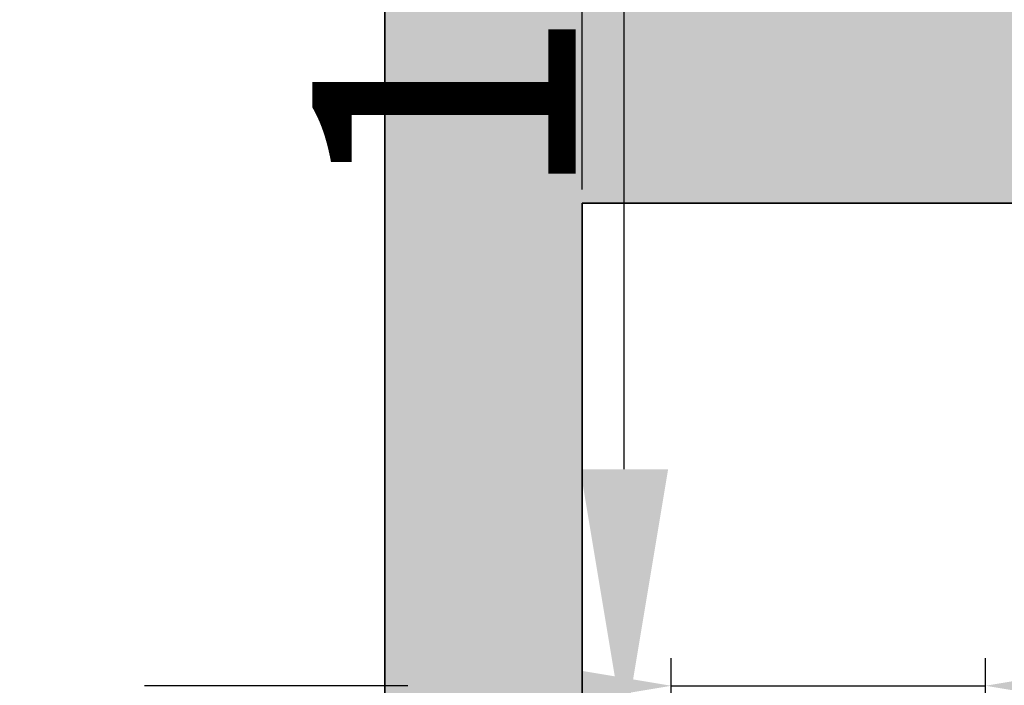
# Model space of a CAD drawing. Units: inches. Extents: x 2083 to 3317, y 1141 to 2115.
# Tile 16 of 256: x 2210 to 2255, y 1447 to 1477. Entities that reach past the tile are written whole.
import ezdxf

# ---------------------------------------------------------------- set-up
doc = ezdxf.new("R2010")
doc.units = ezdxf.units.IN
doc.layers.add('A-ANNO-DIMS', color=2, linetype='Continuous', lineweight=18)
doc.layers.add('A-WALL', color=7, linetype='Continuous', lineweight=35)
doc.layers.add('A-WALL-PATT', color=251, linetype='Continuous', lineweight=13, true_color=0x636466)
doc.styles.get("Standard").update_dxf_attribs({"font": 'arial.ttf'})
doc.dimstyles.new('ISO-25', dxfattribs={"dimtxt": 12, "dimasz": 12, "dimexe": 1.25, "dimexo": 0.625, "dimtad": 1, "dimlunit": 3, "dimtxsty": 'Standard', "dimcen": 2.5, "dimadec": 0, "dimazin": 0, "dimtfac": 1, "dimtmove": 0, "dimatfit": 3, "dimfxl": 1, "dimarcsym": 0})

# ---------------------------------------------------------------- blocks, each defined once
blk = doc.blocks.new('*D13')
at = {"layer": 'A-ANNO-DIMS', "color": 0, "lineweight": -2, "transparency": 16777216}
for p, q in [((2226.335, 1477.761), (2191.976, 1477.761)), ((2193.226, 1465.761), (2193.226, 1275.261)), ((2226.335, 1263.261), (2191.976, 1263.261))]:
    blk.add_line(p, q, dxfattribs=at)
at = {"layer": 'A-ANNO-DIMS', "color": 0, "transparency": 16777216}
for points in [[(2191.226, 1465.761), (2195.226, 1465.761), (2193.226, 1477.761)], [(2191.226, 1275.261), (2195.226, 1275.261), (2193.226, 1263.261)]]:
    blk.add_solid(points, dxfattribs=at)
at = {"layer": 'Defpoints', "color": 0, "transparency": 16777216}
for p in [(2226.96, 1477.761), (2193.226, 1263.261), (2226.96, 1263.261)]:
    blk.add_point(p, dxfattribs=at)
at = {"layer": 'A-ANNO-DIMS', "color": 0, "transparency": 16777216, "insert": (2186.474, 1370.511), "char_height": 12, "attachment_point": 5, "rotation": 90}
blk.add_mtext('17\'-10.5"', dxfattribs=at)
blk = doc.blocks.new('*D30')
at = {"layer": 'A-ANNO-DIMS', "color": 0, "lineweight": -2, "transparency": 16777216}
for p, q in [((2240.018, 1445.274), (2240.018, 1448.046)), ((2254.329, 1445.274), (2254.329, 1448.046)), ((2228.018, 1446.796), (2216.018, 1446.796)), ((2240.018, 1446.796), (2254.329, 1446.796)), ((2266.329, 1446.796), (2413.765, 1446.796))]:
    blk.add_line(p, q, dxfattribs=at)
at = {"layer": 'A-ANNO-DIMS', "color": 0, "transparency": 16777216}
for points in [[(2228.018, 1448.796), (2228.018, 1444.796), (2240.018, 1446.796)], [(2266.329, 1448.796), (2266.329, 1444.796), (2254.329, 1446.796)]]:
    blk.add_solid(points, dxfattribs=at)
at = {"layer": 'Defpoints', "color": 0, "transparency": 16777216}
for p in [(2254.329, 1446.796), (2240.018, 1444.649), (2254.329, 1444.649)]:
    blk.add_point(p, dxfattribs=at)
at = {"layer": 'A-ANNO-DIMS', "color": 0, "transparency": 16777216, "insert": (2346.047, 1453.625), "char_height": 12, "attachment_point": 5}
blk.add_mtext('WC 1\'-2 1/2" TYP.', dxfattribs=at)
blk = doc.blocks.new('*D31')
at = {"layer": 'A-ANNO-DIMS', "color": 0, "lineweight": -2, "transparency": 16777216}
for p, q in [((2237.871, 1456.649), (2237.871, 1541.915)), ((2239.393, 1444.649), (2236.621, 1444.649)), ((2237.871, 1431.548), (2237.871, 1444.649)), ((2239.393, 1431.548), (2236.621, 1431.548)), ((2237.871, 1419.548), (2237.871, 1407.548))]:
    blk.add_line(p, q, dxfattribs=at)
at = {"layer": 'A-ANNO-DIMS', "color": 0, "transparency": 16777216}
for points in [[(2235.871, 1456.649), (2239.871, 1456.649), (2237.871, 1444.649)], [(2235.871, 1419.548), (2239.871, 1419.548), (2237.871, 1431.548)]]:
    blk.add_solid(points, dxfattribs=at)
at = {"layer": 'Defpoints', "color": 0, "transparency": 16777216}
for p in [(2237.871, 1444.649), (2240.018, 1444.649), (2240.018, 1431.548)]:
    blk.add_point(p, dxfattribs=at)
at = {"layer": 'A-ANNO-DIMS', "color": 0, "transparency": 16777216, "insert": (2231.217, 1505.282), "char_height": 12, "attachment_point": 5, "rotation": 90}
blk.add_mtext('1\'-1" TYP.', dxfattribs=at)
blk = doc.blocks.new('*D62')
at = {"layer": 'A-ANNO-DIMS', "color": 0, "lineweight": -2, "transparency": 16777216}
for p, q in [((2235.96, 1469.386), (2235.96, 1522.361)), ((2379.96, 1469.386), (2379.96, 1522.361)), ((2247.96, 1521.111), (2367.96, 1521.111))]:
    blk.add_line(p, q, dxfattribs=at)
at = {"layer": 'A-ANNO-DIMS', "color": 0, "transparency": 16777216}
for points in [[(2247.96, 1523.111), (2247.96, 1519.111), (2235.96, 1521.111)], [(2367.96, 1523.111), (2367.96, 1519.111), (2379.96, 1521.111)]]:
    blk.add_solid(points, dxfattribs=at)
at = {"layer": 'Defpoints', "color": 0, "transparency": 16777216}
for p in [(2379.96, 1521.111), (2235.96, 1468.761), (2379.96, 1468.761)]:
    blk.add_point(p, dxfattribs=at)
at = {"layer": 'A-ANNO-DIMS', "color": 0, "transparency": 16777216, "insert": (2307.96, 1527.863), "char_height": 12, "attachment_point": 5}
blk.add_mtext('12\'-0"', dxfattribs=at)

msp = doc.modelspace()

# ---------------------------------------------------------------- hatches: boundary and pattern name
at = {"layer": 'A-WALL-PATT'}
h = msp.add_hatch(color=256, dxfattribs=at)
h.dxf.hatch_style = 1
h.paths.add_polyline_path([(3126.96, 2020.761), (2748.96, 2020.761), (2604.96, 2020.761), (2226.96, 2020.761), (2226.96, 1702.761), (2466.96, 1702.761), (2466.96, 1582.761), (2418.96, 1582.761), (2418.96, 1477.761), (2226.96, 1477.761), (2226.96, 1263.261), (2544.96, 1263.261), (2544.96, 1411.761), (2604.96, 1411.761), (2685.96, 1411.761), (2685.96, 1420.761), (2604.96, 1420.761), (2604.96, 1573.761), (2604.96, 1702.761), (2604.96, 2011.761), (2748.96, 2011.761), (2748.96, 1702.761), (2862.96, 1702.761), (2862.96, 1621.761), (2871.96, 1621.761), (2871.96, 1702.761), (2883.96, 1702.761), (2883.96, 1706.939, -0.026459), (2883.96, 1711.761), (2757.96, 1711.761), (2757.96, 1807.761), (2787.96, 1807.761), (2787.96, 1812.261), (2757.96, 1812.261), (2757.96, 2011.761), (2877.96, 2011.761), (2877.96, 1812.261), (2847.96, 1812.261), (2847.96, 1807.761), (2889.836, 1807.761), (2889.836, 1812.261), (2882.46, 1812.261), (2882.46, 2011.761), (3117.96, 2011.761), (3117.96, 1812.261), (2937.836, 1812.261), (2937.836, 1807.761), (2995.71, 1807.761), (2995.71, 1796.118), (3000.21, 1796.118), (3000.21, 1807.761), (3117.96, 1807.761), (3117.96, 1711.761), (3000.21, 1711.761), (3000.21, 1760.118), (2998.573, 1760.118, -0.020711), (2995.71, 1760.118), (2995.71, 1711.761), (2931.96, 1711.761), (2931.96, 1702.761), (3126.96, 1702.761)])
h.paths.add_polyline_path([(2471.46, 2011.761), (2471.46, 1810.011), (2462.717, 1810.011), (2462.717, 1805.511), (2505.96, 1805.511), (2505.96, 1810.011), (2475.96, 1810.011), (2475.96, 2011.761), (2595.96, 2011.761), (2595.96, 1810.011), (2565.96, 1810.011), (2565.96, 1805.511), (2595.96, 1805.511), (2595.96, 1711.761), (2235.96, 1711.761), (2235.96, 1805.511), (2353.71, 1805.511), (2353.71, 1796.054), (2358.21, 1796.054), (2358.21, 1805.511), (2414.717, 1805.511), (2414.717, 1810.011), (2235.96, 1810.011), (2235.96, 2011.761)], flags=16)
h.paths.add_polyline_path([(2270.205, 1994.61), (2270.205, 1970.61), (2246.205, 1970.61), (2246.205, 1994.61)], flags=0)
edge = h.paths.add_edge_path(flags=0)
edge.add_ellipse((2332.027, 1899.798), major_axis=(-3.043, 3.043), ratio=0.168252, start_angle=-161.3322, end_angle=-156.3071, ccw=False)
edge.add_ellipse((2333.082, 1898.744), major_axis=(-1.055, 1.055), ratio=0.453532, start_angle=-123.371, end_angle=-94.1591)
edge = h.paths.add_edge_path(flags=0)
edge.add_ellipse((2332.027, 1968.876), major_axis=(3.043, 3.043), ratio=0.168252, start_angle=18.6678, end_angle=23.6929)
edge.add_spline(control_points=[(2332.926, 1970.691), (2332.227, 1970.336), (2330.894, 1969.659), (2328.413, 1970.932), (2327.204, 1967.749), (2324.71, 1969.956), (2322.533, 1967.012), (2320.013, 1971.296), (2317.68, 1968.158), (2316.041, 1967.102), (2315.427, 1966.81)], knot_values=[0, 0, 0, 0, 2.267059, 4.324559, 6.685584, 8.878641, 11.121502, 14.300359, 17.755284, 19.732645, 19.732645, 19.732645, 19.732645], degree=3, periodic=0)
edge.add_ellipse((2332.027, 1968.876), major_axis=(3.043, 3.043), ratio=0.168252, start_angle=18.6678, end_angle=23.6929, ccw=False)
edge.add_ellipse((2333.082, 1969.931), major_axis=(1.055, 1.055), ratio=0.453532, start_angle=56.629, end_angle=85.8409, ccw=False)
edge = h.paths.add_edge_path(flags=0)
edge.add_spline(control_points=[(2296.428, 1967.988), (2293.628, 1965.336), (2287.704, 1959.727), (2299.744, 1949.996), (2294.533, 1935.669), (2290.573, 1920.604), (2293.394, 1909.974), (2296.185, 1904.967)], knot_values=[0.099185, 0.099185, 0.099185, 0.099185, 0.345301, 0.619822, 0.982653, 1.386093, 1.810555, 1.810555, 1.810555, 1.810555], degree=3, periodic=0)
edge.add_spline(control_points=[(2296.185, 1904.967), (2297.384, 1902.619), (2298.001, 1901.949), (2298.553, 1901.468)], knot_values=[0.006246, 0.006246, 0.006246, 0.006246, 0.055476, 0.055476, 0.055476, 0.055476], degree=3, periodic=0)
edge.add_spline(control_points=[(2298.553, 1901.468), (2297.259, 1900.923), (2295.225, 1900.232), (2293.06, 1900.614), (2292.101, 1900.788), (2292.09, 1900.791)], knot_values=[0.312835, 0.312835, 0.312835, 0.312835, 0.40178, 0.474987, 0.475903, 0.475903, 0.475903, 0.475903], degree=3, periodic=0)
edge.add_arc((2292.794, 1904.664), 3.937, 215.4209, 259.6982, ccw=False)
edge.add_spline(control_points=[(2289.585, 1902.382), (2289.477, 1902.535), (2289.368, 1902.688), (2289.261, 1902.841)], knot_values=[0.102872, 0.102872, 0.102872, 0.102872, 0.116896, 0.116896, 0.116896, 0.116896], degree=3, periodic=0)
edge.add_spline(control_points=[(2289.261, 1902.841), (2288.687, 1902.55), (2287.64, 1902.02), (2285.881, 1901.874), (2283.853, 1901.504), (2281.72, 1899.711), (2278.467, 1899.493), (2276.157, 1901.883), (2272.259, 1899.804), (2267.778, 1901.843), (2262.244, 1900.184), (2257.415, 1901.782), (2254.318, 1900.726), (2253.178, 1900.337)], knot_values=[0, 0, 0, 0, 1.907977, 3.477176, 5.261074, 7.972851, 11.680248, 13.717921, 16.939592, 22.789562, 27.502503, 33.595215, 37.145618, 37.145618, 37.145618, 37.145618], degree=3, periodic=0)
edge.add_line((2253.178, 1900.337), (2250.244, 1902.841))
edge.add_line((2250.244, 1902.841), (2250.244, 1965.833))
edge.add_line((2250.244, 1965.833), (2253.178, 1968.337))
edge.add_spline(control_points=[(2253.178, 1968.337), (2254.318, 1967.948), (2257.415, 1966.892), (2262.244, 1968.49), (2267.778, 1966.831), (2271.527, 1968.537), (2273.876, 1967.828), (2274.207, 1967.728)], knot_values=[0, 0, 0, 0, 0.09018, 0.244935, 0.364644, 0.513233, 0.537855, 0.537855, 0.537855, 0.537855], degree=3, periodic=0)
edge.add_arc((2274.353, 1963.793), 3.937, 72.0511, 92.1279, ccw=False)
edge.add_arc((2281.297, 1985.23), 18.596, 252.0511, 288.5657)
edge.add_arc((2292.317, 1956.029), 12.646, 71.0268, 113.7782, ccw=False)
edge = h.paths.add_edge_path(flags=0)
edge.add_spline(control_points=[(2274.899, 1951.856), (2275.066, 1951.617), (2275.233, 1951.377), (2275.398, 1951.136)], knot_values=[1.409916, 1.409916, 1.409916, 1.409916, 1.43159, 1.43159, 1.43159, 1.43159], degree=3, periodic=0)
edge.add_spline(control_points=[(2275.398, 1951.136), (2275.792, 1950.562), (2276.179, 1949.984), (2276.546, 1949.397)], knot_values=[1.358238, 1.358238, 1.358238, 1.358238, 1.409916, 1.409916, 1.409916, 1.409916], degree=3, periodic=0)
edge.add_line((2276.546, 1949.397), (2277.437, 1947.862))
edge.add_spline(control_points=[(2277.437, 1947.862), (2276.304, 1945.673), (2274.64, 1942.427), (2274.632, 1938.094), (2272.799, 1930.852), (2274.356, 1943.897), (2275.948, 1947.923), (2276.546, 1949.397)], knot_values=[0.005632, 0.005632, 0.005632, 0.005632, 0.186014, 0.266002, 0.357087, 0.59639, 0.739732, 0.739732, 0.739732, 0.739732], degree=3, periodic=0)
edge.add_spline(control_points=[(2276.546, 1949.397), (2276.179, 1949.984), (2275.792, 1950.562), (2275.398, 1951.136)], knot_values=[1.358238, 1.358238, 1.358238, 1.358238, 1.409916, 1.409916, 1.409916, 1.409916], degree=3, periodic=0)
edge.add_spline(control_points=[(2275.398, 1951.136), (2274.943, 1950.08), (2274.208, 1948.025), (2273.935, 1944.851), (2272.469, 1937.627), (2273.466, 1945.696), (2274.701, 1951.059), (2274.899, 1951.856)], knot_values=[0.104364, 0.104364, 0.104364, 0.104364, 0.189636, 0.269624, 0.36071, 0.600013, 0.644622, 0.644622, 0.644622, 0.644622], degree=3, periodic=0)
h.paths.add_polyline_path([(2269.168, 1963.128, -0.357527), (2268.171, 1960.976, -0.092561), (2268.171, 1939.436, -0.357527), (2269.168, 1937.285, -0.357527), (2267.016, 1938.282, -0.164785), (2254.686, 1938.282, -0.357527), (2252.534, 1937.285, -0.357527), (2253.531, 1939.436, -0.092561), (2253.531, 1960.976, -0.357527), (2252.534, 1963.128, -0.357527), (2254.686, 1962.131, -0.164785), (2267.016, 1962.131, -0.357527)], flags=0)
h.paths.add_polyline_path([(2248.874, 1967.802), (2248.874, 1957.028), (2249.458, 1957.028), (2249.458, 1911.647), (2248.874, 1911.647), (2248.874, 1900.873), (2246.512, 1900.873, 0.197327), (2244.15, 1902.457), (2244.15, 1966.218, 0.197327), (2246.512, 1967.802)], flags=0)
h.paths.add_polyline_path([(2269.168, 1931.389, -0.357527), (2268.171, 1929.238, -0.092561), (2268.171, 1907.698, -0.357527), (2269.168, 1905.547, -0.357527), (2267.016, 1906.544, -0.164785), (2254.686, 1906.544, -0.357527), (2252.534, 1905.547, -0.357527), (2253.531, 1907.698, -0.092561), (2253.531, 1929.238, -0.357527), (2252.534, 1931.389, -0.357527), (2254.686, 1930.392, -0.164785), (2267.016, 1930.392, -0.357527)], flags=0)
edge = h.paths.add_edge_path(flags=0)
edge.add_spline(control_points=[(2276.197, 1906.724), (2276.168, 1909.029), (2276.114, 1913.372), (2270.598, 1924.925), (2273.905, 1919.013), (2275.922, 1916.262), (2275.475, 1912.402), (2277.258, 1910.381), (2276.696, 1908.225), (2276.646, 1906.813), (2276.618, 1906.008)], knot_values=[0, 0, 0, 0, 8.61026, 16.221274, 18.843057, 23.804898, 27.440828, 29.356102, 31.203478, 33.650687, 33.650687, 33.650687, 33.650687], degree=3, periodic=0)
edge.add_spline(control_points=[(2276.618, 1906.008), (2276.623, 1905.624), (2276.498, 1904.629), (2275.442, 1903.855), (2274.937, 1903.08), (2274.859, 1902.841)], knot_values=[0.156488, 0.156488, 0.156488, 0.156488, 0.184398, 0.231376, 0.250598, 0.250598, 0.250598, 0.250598], degree=3, periodic=0)
edge.add_line((2274.859, 1902.841), (2276.506, 1902.841))
edge.add_spline(control_points=[(2276.506, 1902.841), (2276.788, 1903.085), (2277.665, 1904.125), (2278.25, 1904.341), (2277.654, 1908.527), (2278.156, 1906.228), (2278.1, 1905.286), (2278.847, 1904.069), (2277.857, 1903.415), (2277.874, 1902.991), (2277.904, 1902.841)], knot_values=[0.059574, 0.059574, 0.059574, 0.059574, 0.080753, 0.103741, 0.16972, 0.176036, 0.207137, 0.240474, 0.262341, 0.27366, 0.27366, 0.27366, 0.27366], degree=3, periodic=0)
edge.add_line((2277.904, 1902.841), (2280.03, 1902.841))
edge.add_spline(control_points=[(2280.03, 1902.841), (2279.888, 1903.088), (2279.499, 1903.982), (2280.152, 1905.939), (2278.104, 1909.658), (2279.762, 1907.185), (2280.328, 1904.875), (2280.485, 1903.49), (2281.463, 1903.249), (2281.758, 1902.936), (2281.834, 1902.841)], knot_values=[0.013856, 0.013856, 0.013856, 0.013856, 0.034874, 0.088867, 0.107879, 0.126738, 0.158714, 0.193757, 0.217487, 0.226722, 0.226722, 0.226722, 0.226722], degree=3, periodic=0)
edge.add_spline(control_points=[(2281.834, 1902.841), (2281.788, 1902.827), (2281.647, 1902.783), (2281.396, 1902.859), (2281.088, 1902.985), (2280.721, 1903.061), (2280.333, 1903.026), (2280.125, 1902.899), (2280.03, 1902.841)], knot_values=[0, 0, 0, 0, 0.14413, 0.435517, 0.749276, 1.153046, 1.548371, 1.878348, 1.878348, 1.878348, 1.878348], degree=3, periodic=0)
edge.add_line((2280.03, 1902.841), (2277.904, 1902.841))
edge.add_spline(control_points=[(2277.904, 1902.841), (2277.893, 1902.796), (2277.865, 1902.68), (2277.607, 1902.687), (2277.274, 1902.801), (2276.838, 1902.62), (2276.584, 1902.789), (2276.506, 1902.841)], knot_values=[0, 0, 0, 0, 0.127189, 0.326199, 0.628009, 1.24357, 1.515331, 1.515331, 1.515331, 1.515331], degree=3, periodic=0)
edge.add_line((2276.506, 1902.841), (2274.859, 1902.841))
edge.add_spline(control_points=[(2274.859, 1902.841), (2274.814, 1902.899), (2274.725, 1903.013), (2274.493, 1903.119), (2274.244, 1902.961), (2273.937, 1903.185), (2273.614, 1902.983), (2273.408, 1902.883), (2273.322, 1902.841)], knot_values=[0, 0, 0, 0, 0.21843, 0.436957, 0.687977, 0.990379, 1.398396, 1.69185, 1.69185, 1.69185, 1.69185], degree=3, periodic=0)
edge.add_spline(control_points=[(2273.322, 1902.841), (2273.617, 1903.446), (2274.274, 1904.538), (2276.027, 1904.574), (2276.207, 1906.584), (2276.197, 1906.724)], knot_values=[0.012227, 0.012227, 0.012227, 0.012227, 0.059472, 0.106218, 0.134458, 0.134458, 0.134458, 0.134458], degree=3, periodic=0)
h.paths.add_polyline_path([(2270.776, 1897.79), (2270.776, 1873.79), (2246.776, 1873.79), (2246.776, 1897.79)], flags=0)
h.paths.add_polyline_path([(2353.71, 1760.005), (2353.71, 1760.054), (2358.21, 1760.054, -0.033729)], flags=0)
h.paths.add_polyline_path([(2321.819, 1737.529), (2341.995, 1737.529, -0.414214), (2343.203, 1736.321), (2343.203, 1721.021, -0.414214), (2341.995, 1719.813), (2321.819, 1719.813, -0.414214), (2320.611, 1721.021), (2320.611, 1736.321, -0.414214)], flags=0)
h.paths.add_polyline_path([(2324.235, 1736.321), (2339.579, 1736.321, -0.414214), (2341.995, 1733.905), (2341.995, 1725.45, -0.414214), (2339.579, 1723.034), (2333.681, 1723.034), (2333.845, 1722.045, -0.870646), (2335.425, 1721.826, -0.767327), (2333.923, 1721.423), (2331.291, 1721.423, -0.767327), (2329.788, 1721.826, -0.870646), (2331.368, 1722.045), (2331.533, 1723.034), (2324.235, 1723.034, -0.414214), (2321.819, 1725.45), (2321.819, 1733.905, -0.414214)], flags=0)
h.paths.add_polyline_path([(2570.484, 1928.615), (2589.684, 1928.615), (2590.169, 1928.615), (2590.169, 1904.993), (2570.484, 1904.993)], flags=0)
h.paths.add_polyline_path([(2574.447, 1927.264, -1), (2572.829, 1927.264, -1)], flags=0)
h.paths.add_polyline_path([(2573.09, 1926.941), (2573.925, 1927.776), (2574.148, 1927.553), (2573.313, 1926.718)], flags=0)
h.paths.add_polyline_path([(2578.779, 1919.73, -1), (2571.592, 1919.73, -1)], flags=0)
h.paths.add_polyline_path([(2578.385, 1919.73, -1), (2571.985, 1919.73, -1)], flags=0)
h.paths.add_polyline_path([(2331.596, 1729.476, -1), (2333.618, 1729.476, -1)], flags=0)
h.paths.add_polyline_path([(2578.034, 1927.264, -1), (2576.416, 1927.264, -1)], flags=0)
h.paths.add_polyline_path([(2576.689, 1927.531), (2576.912, 1927.754), (2577.747, 1926.919), (2577.524, 1926.696)], flags=0)
h.paths.add_polyline_path([(2578.139, 1909.86, -1), (2572.232, 1909.86, -1)], flags=0)
h.paths.add_polyline_path([(2577.745, 1909.86, -1), (2572.625, 1909.86, -1)], flags=0)
h.paths.add_polyline_path([(2583.798, 1927.264, -1), (2582.179, 1927.264, -1)], flags=0)
h.paths.add_polyline_path([(2582.719, 1927.754), (2583.554, 1926.919), (2583.331, 1926.696), (2582.496, 1927.531)], flags=0)
h.paths.add_polyline_path([(2582.496, 1927.531), (2582.719, 1927.754), (2583.554, 1926.919), (2583.331, 1926.696)], flags=0)
h.paths.add_polyline_path([(2587.739, 1920.53, -1), (2581.832, 1920.53, -1)], flags=0)
h.paths.add_polyline_path([(2587.345, 1920.53, -1), (2582.225, 1920.53, -1)], flags=0)
h.paths.add_polyline_path([(2587.385, 1927.264, -1), (2585.766, 1927.264, -1)], flags=0)
h.paths.add_polyline_path([(2586.082, 1926.98), (2586.917, 1927.815), (2587.14, 1927.593), (2586.305, 1926.758)], flags=0)
h.paths.add_polyline_path([(2588.379, 1910.66, -1), (2581.192, 1910.66, -1)], flags=0)
h.paths.add_polyline_path([(2587.985, 1910.66, -1), (2581.585, 1910.66, -1)], flags=0)
h.paths.add_polyline_path([(2417.168, 1729.478), (2437.344, 1729.478, -0.414214), (2438.552, 1728.27), (2438.552, 1712.969, -0.414214), (2437.344, 1711.761), (2417.168, 1711.761, -0.414214), (2415.96, 1712.969), (2415.96, 1728.27, -0.414214)], flags=0)
h.paths.add_polyline_path([(2419.584, 1728.27), (2434.928, 1728.27, -0.414214), (2437.344, 1725.854), (2437.344, 1717.398, -0.414214), (2434.928, 1714.983), (2429.029, 1714.983), (2429.194, 1713.994, -0.870646), (2430.774, 1713.775, -0.767327), (2429.271, 1713.372), (2426.64, 1713.372, -0.767327), (2425.137, 1713.775, -0.870646), (2426.717, 1713.994), (2426.882, 1714.983), (2419.584, 1714.983, -0.414214), (2417.168, 1717.398), (2417.168, 1725.854, -0.414214)], flags=0)
h.paths.add_polyline_path([(2419.584, 1728.27), (2434.928, 1728.27, -0.414214), (2437.344, 1725.854), (2437.344, 1717.398, -0.414214), (2434.928, 1714.983), (2429.029, 1714.983), (2428.358, 1719.009), (2427.553, 1719.009), (2426.882, 1714.983), (2419.584, 1714.983, -0.414214), (2417.168, 1717.398), (2417.168, 1725.854, -0.414214)], flags=0)
h.paths.add_polyline_path([(2426.944, 1721.425, -1), (2428.967, 1721.425, -1)], flags=0)
h.paths.add_polyline_path([(2475.96, 1702.761), (2595.96, 1702.761), (2595.96, 1582.761), (2475.96, 1582.761)], flags=16)
h.paths.add_polyline_path([(2427.96, 1573.761), (2595.96, 1573.761), (2595.96, 1468.761), (2595.96, 1420.761), (2384.46, 1420.761), (2384.46, 1468.761), (2427.96, 1468.761)], flags=16)
h.paths.add_polyline_path([(2379.96, 1468.761), (2379.96, 1420.761), (2235.96, 1420.761), (2235.96, 1468.761)], flags=16)
h.paths.add_polyline_path([(2317.816, 1466.696), (2337.992, 1466.696, -0.414214), (2339.2, 1465.488), (2339.2, 1450.187, -0.414214), (2337.992, 1448.979), (2317.816, 1448.979, -0.414214), (2316.608, 1450.187), (2316.608, 1465.488, -0.414214)], flags=0)
h.paths.add_polyline_path([(2320.232, 1465.488), (2335.576, 1465.488, -0.414214), (2337.992, 1463.072), (2337.992, 1454.616, -0.414214), (2335.576, 1452.2), (2329.677, 1452.2), (2329.842, 1451.212, -0.870646), (2331.422, 1450.992, -0.767327), (2329.92, 1450.59), (2327.288, 1450.59, -0.767327), (2325.785, 1450.992, -0.870646), (2327.365, 1451.212), (2327.53, 1452.2), (2320.232, 1452.2, -0.414214), (2317.816, 1454.616), (2317.816, 1463.072, -0.414214)], flags=0)
h.paths.add_polyline_path([(2320.232, 1465.488), (2335.576, 1465.488, -0.414214), (2337.992, 1463.072), (2337.992, 1454.616, -0.414214), (2335.576, 1452.2), (2329.677, 1452.2), (2329.006, 1456.227), (2328.201, 1456.227), (2327.53, 1452.2), (2320.232, 1452.2, -0.414214), (2317.816, 1454.616), (2317.816, 1463.072, -0.414214)], flags=0)
h.paths.add_polyline_path([(2327.593, 1458.643, -1), (2329.615, 1458.643, -1)], flags=0)
h.paths.add_polyline_path([(2244.412, 1433.34), (2241.921, 1433.34, -0.414214), (2240.018, 1435.244), (2240.018, 1440.953, -0.414211), (2241.921, 1442.856), (2244.412, 1442.856, -1.976472)], flags=0)
h.paths.add_polyline_path([(2245.357, 1434.398, -0.414214), (2245.357, 1441.799, -2.144098)], flags=0)
h.paths.add_polyline_path([(2535.96, 1416.261), (2535.96, 1272.261), (2235.96, 1272.261), (2235.96, 1416.261)], flags=16)
h.paths.add_polyline_path([(2260.12, 1384.293), (2260.12, 1362.039), (2237.865, 1362.039), (2237.865, 1384.293)], flags=0)
edge = h.paths.add_edge_path(flags=0)
edge.add_line((2318.252, 1362.093), (2318.146, 1362.001))
edge.add_ellipse((2317.445, 1360.431), major_axis=(2.822, 2.822), ratio=0.168252, start_angle=18.6678, end_angle=20.9481, ccw=False)
edge.add_ellipse((2318.423, 1361.409), major_axis=(0.978, 0.978), ratio=0.453532, start_angle=56.629, end_angle=70.2262, ccw=False)
edge = h.paths.add_edge_path(flags=0)
edge.add_line((2319.107, 1295.571), (2319.015, 1295.677))
edge.add_ellipse((2317.445, 1296.378), major_axis=(-2.822, 2.822), ratio=0.168252, start_angle=-161.3322, end_angle=-159.0519, ccw=False)
edge.add_ellipse((2318.423, 1295.4), major_axis=(-0.978, 0.978), ratio=0.453532, start_angle=-123.371, end_angle=-109.7738)
edge = h.paths.add_edge_path(flags=0)
edge.add_spline(control_points=[(2284.21, 1301.17), (2284.581, 1300.445), (2284.891, 1299.892), (2285.16, 1299.461)], knot_values=[0.039066, 0.039066, 0.039066, 0.039066, 0.055476, 0.055476, 0.055476, 0.055476], degree=3, periodic=0)
edge.add_line((2285.16, 1299.461), (2284.21, 1301.17))
edge = h.paths.add_edge_path(flags=0)
edge.add_line((2280.412, 1297.298), (2283.37, 1297.036))
edge.add_line((2283.37, 1297.036), (2286.406, 1297.926))
edge.add_spline(control_points=[(2286.406, 1297.926), (2285.305, 1297.463), (2284.345, 1297.129), (2283.37, 1297.036)], knot_values=[0.394369, 0.394369, 0.394369, 0.394369, 0.475903, 0.475903, 0.475903, 0.475903], degree=3, periodic=0)
edge.add_spline(control_points=[(2283.37, 1297.036), (2283.281, 1297.028), (2282.316, 1296.957), (2281.313, 1297.134), (2280.423, 1297.296), (2280.412, 1297.298)], knot_values=[0.312835, 0.312835, 0.312835, 0.312835, 0.320246, 0.393453, 0.394369, 0.394369, 0.394369, 0.394369], degree=3, periodic=0)
edge = h.paths.add_edge_path(flags=0)
edge.add_line((2284.436, 1359.607), (2280.446, 1355.328))
edge.add_line((2280.446, 1355.328), (2279.58, 1351.018))
edge.add_line((2279.58, 1351.018), (2282.413, 1346.58))
edge.add_spline(control_points=[(2282.413, 1346.58), (2283.153, 1345.589), (2284.253, 1344.029), (2284.801, 1342.387), (2284.935, 1341.806)], knot_values=[1.240098, 1.240098, 1.240098, 1.240098, 1.332892, 1.382712, 1.382712, 1.382712, 1.382712], degree=3, periodic=0)
edge.add_spline(control_points=[(2284.935, 1341.806), (2285.319, 1340.141), (2285.233, 1338.409), (2284.91, 1336.654)], knot_values=[1.097484, 1.097484, 1.097484, 1.097484, 1.240098, 1.240098, 1.240098, 1.240098], degree=3, periodic=0)
edge.add_spline(control_points=[(2284.91, 1336.654), (2284.587, 1334.899), (2284.027, 1333.12), (2283.463, 1331.361)], knot_values=[0.95487, 0.95487, 0.95487, 0.95487, 1.097484, 1.097484, 1.097484, 1.097484], degree=3, periodic=0)
edge.add_line((2283.463, 1331.361), (2281.89, 1326.153))
edge.add_line((2281.89, 1326.153), (2280.756, 1321.056))
edge.add_line((2280.756, 1321.056), (2280.299, 1316.002))
edge.add_line((2280.299, 1316.002), (2280.716, 1310.95))
edge.add_line((2280.716, 1310.95), (2282.028, 1305.972))
edge.add_line((2282.028, 1305.972), (2284.21, 1301.17))
edge.add_spline(control_points=[(2284.21, 1301.17), (2283.341, 1302.73), (2282.612, 1304.336), (2282.028, 1305.972)], knot_values=[0.099185, 0.099185, 0.099185, 0.099185, 0.241799, 0.241799, 0.241799, 0.241799], degree=3, periodic=0)
edge.add_spline(control_points=[(2282.028, 1305.972), (2281.444, 1307.608), (2281.005, 1309.273), (2280.716, 1310.95)], knot_values=[0.241799, 0.241799, 0.241799, 0.241799, 0.384413, 0.384413, 0.384413, 0.384413], degree=3, periodic=0)
edge.add_spline(control_points=[(2280.716, 1310.95), (2280.433, 1312.588), (2280.289, 1314.277), (2280.299, 1315.962), (2280.299, 1316.002)], knot_values=[0.384413, 0.384413, 0.384413, 0.384413, 0.523647, 0.527028, 0.527028, 0.527028, 0.527028], degree=3, periodic=0)
edge.add_spline(control_points=[(2280.299, 1316.002), (2280.312, 1317.687), (2280.478, 1319.368), (2280.756, 1321.056)], knot_values=[0.527028, 0.527028, 0.527028, 0.527028, 0.669642, 0.669642, 0.669642, 0.669642], degree=3, periodic=0)
edge.add_spline(control_points=[(2280.756, 1321.056), (2281.035, 1322.744), (2281.426, 1324.44), (2281.89, 1326.153)], knot_values=[0.669642, 0.669642, 0.669642, 0.669642, 0.812256, 0.812256, 0.812256, 0.812256], degree=3, periodic=0)
edge.add_spline(control_points=[(2281.89, 1326.153), (2282.264, 1327.533), (2282.788, 1329.262), (2283.353, 1331.018), (2283.463, 1331.361)], knot_values=[0.812256, 0.812256, 0.812256, 0.812256, 0.927087, 0.95487, 0.95487, 0.95487, 0.95487], degree=3, periodic=0)
edge.add_line((2283.463, 1331.361), (2284.91, 1336.654))
edge.add_line((2284.91, 1336.654), (2284.935, 1341.806))
edge.add_line((2284.935, 1341.806), (2282.413, 1346.58))
edge.add_spline(control_points=[(2282.413, 1346.58), (2281.275, 1348.104), (2280.078, 1349.57), (2279.58, 1351.018)], knot_values=[1.382712, 1.382712, 1.382712, 1.382712, 1.525326, 1.525326, 1.525326, 1.525326], degree=3, periodic=0)
edge.add_spline(control_points=[(2279.58, 1351.018), (2279.443, 1351.415), (2279.136, 1352.857), (2279.735, 1354.29), (2280.446, 1355.328)], knot_values=[1.525326, 1.525326, 1.525326, 1.525326, 1.564439, 1.667941, 1.667941, 1.667941, 1.667941], degree=3, periodic=0)
edge.add_spline(control_points=[(2280.446, 1355.328), (2281.426, 1356.758), (2282.931, 1358.183), (2284.436, 1359.607)], knot_values=[1.667941, 1.667941, 1.667941, 1.667941, 1.810555, 1.810555, 1.810555, 1.810555], degree=3, periodic=0)
edge.add_arc((2280.623, 1348.518), 11.726, 71.0268, 113.7782)
edge.add_arc((2270.405, 1375.595), 17.244, 252.0511, 288.5657, ccw=False)
edge.add_arc((2263.966, 1355.718), 3.651, 72.0511, 92.1279)
edge.add_arc((2263.966, 1355.718), 3.651, 92.1279, 177.9851)
edge.add_spline(control_points=[(2260.318, 1355.846), (2260.26, 1354.221), (2260.551, 1350.187), (2262.999, 1346.766), (2264.473, 1344.649)], knot_values=[1.43159, 1.43159, 1.43159, 1.43159, 1.564144, 1.770695, 1.770695, 1.770695, 1.770695], degree=3, periodic=0)
edge.add_line((2264.473, 1344.649), (2264.936, 1343.983))
edge.add_spline(control_points=[(2263.801, 1340.248), (2263.843, 1340.514), (2264.067, 1341.756), (2264.513, 1343.002), (2264.935, 1343.981)], knot_values=[0.53657, 0.53657, 0.53657, 0.53657, 0.559349, 0.644622, 0.644622, 0.644622, 0.644622], degree=3, periodic=0)
edge.add_spline(control_points=[(2264.935, 1343.981), (2265.118, 1343.715), (2265.299, 1343.448), (2265.477, 1343.179)], knot_values=[1.384077, 1.384077, 1.384077, 1.384077, 1.409916, 1.409916, 1.409916, 1.409916], degree=3, periodic=0)
edge.add_spline(control_points=[(2265.477, 1343.179), (2265.655, 1342.911), (2265.829, 1342.641), (2265.999, 1342.369)], knot_values=[1.358238, 1.358238, 1.358238, 1.358238, 1.384077, 1.384077, 1.384077, 1.384077], degree=3, periodic=0)
edge.add_line((2265.999, 1342.369), (2266.826, 1340.946))
edge.add_spline(control_points=[(2266.826, 1340.946), (2268.894, 1337.09), (2271.398, 1325.843), (2270.516, 1310.569), (2275.919, 1301.861), (2277.79, 1299.199)], knot_values=[0.116896, 0.116896, 0.116896, 0.116896, 0.472987, 1.050969, 1.313793, 1.313793, 1.313793, 1.313793], degree=3, periodic=0)
edge.add_spline(control_points=[(2277.79, 1299.199), (2277.839, 1299.128), (2277.889, 1299.057), (2277.94, 1298.987)], knot_values=[0.109884, 0.109884, 0.109884, 0.109884, 0.116896, 0.116896, 0.116896, 0.116896], degree=3, periodic=0)
edge.add_line((2277.94, 1298.987), (2277.789, 1299.199))
edge.add_spline(control_points=[(2277.789, 1299.199), (2277.257, 1298.929), (2276.286, 1298.438), (2275.039, 1298.334), (2274.383, 1298.239), (2274.215, 1298.209)], knot_values=[33.12187, 33.12187, 33.12187, 33.12187, 35.029056, 36.598255, 37.144827, 37.144827, 37.144827, 37.144827], degree=3, periodic=0)
edge.add_line((2274.215, 1298.209), (2273.073, 1297.893))
edge.add_spline(control_points=[(2273.073, 1297.893), (2272.323, 1297.58), (2271.039, 1296.511), (2269.248, 1296.226), (2268.423, 1296.375)], knot_values=[26.532584, 26.532584, 26.532584, 26.532584, 29.198919, 31.839101, 31.839101, 31.839101, 31.839101], degree=3, periodic=0)
edge.add_line((2268.423, 1296.375), (2263.879, 1297.458))
edge.add_spline(control_points=[(2263.879, 1297.458), (2263.556, 1297.359), (2261.86, 1296.839), (2260.239, 1297.282), (2258.933, 1297.516)], knot_values=[15.919551, 15.919551, 15.919551, 15.919551, 16.939592, 21.226067, 21.226067, 21.226067, 21.226067], degree=3, periodic=0)
edge.add_line((2258.933, 1297.516), (2254.055, 1297.329))
edge.add_spline(control_points=[(2254.055, 1297.329), (2253.756, 1297.296), (2252.114, 1297.165), (2250.462, 1297.544), (2249.13, 1297.668)], knot_values=[5.306517, 5.306517, 5.306517, 5.306517, 6.276435, 10.613034, 10.613034, 10.613034, 10.613034], degree=3, periodic=0)
edge.add_line((2249.13, 1297.668), (2244.332, 1296.878))
edge.add_line((2244.332, 1296.878), (2241.611, 1299.199))
edge.add_line((2241.611, 1299.199), (2241.611, 1357.609))
edge.add_line((2241.611, 1357.609), (2244.332, 1359.931))
edge.add_line((2244.332, 1359.931), (2252.729, 1359.543))
edge.add_spline(control_points=[(2252.729, 1359.543), (2252.871, 1359.546), (2253.306, 1359.548), (2253.74, 1359.514), (2254.032, 1359.482)], knot_values=[0.233291, 0.233291, 0.233291, 0.233291, 0.244935, 0.268927, 0.268927, 0.268927, 0.268927], degree=3, periodic=0)
edge.add_line((2254.032, 1359.482), (2259.587, 1359.416))
edge.add_spline(control_points=[(2259.587, 1359.416), (2260.677, 1359.629), (2262.073, 1359.897), (2263.524, 1359.459), (2263.83, 1359.366)], knot_values=[0.422516, 0.422516, 0.422516, 0.422516, 0.513233, 0.537855, 0.537855, 0.537855, 0.537855], degree=3, periodic=0)
edge.add_arc((2263.966, 1355.718), 3.651, 72.0511, 92.1279, ccw=False)
edge.add_arc((2270.405, 1375.595), 17.244, 252.0511, 288.5657)
edge.add_arc((2280.623, 1348.518), 11.726, 71.0268, 113.7782, ccw=False)
h.paths.add_polyline_path([(2240.341, 1359.435), (2240.341, 1349.444), (2240.882, 1349.444), (2240.882, 1307.365), (2240.341, 1307.365), (2240.341, 1297.374), (2238.15, 1297.374, 0.197327), (2235.96, 1298.843), (2235.96, 1357.966, 0.197327), (2238.15, 1359.435)], flags=0)
h.paths.add_polyline_path([(2259.158, 1355.101, -0.357527), (2258.233, 1353.106, -0.092561), (2258.233, 1333.133, -0.357527), (2259.158, 1331.138, -0.357527), (2257.163, 1332.062, -0.164785), (2245.729, 1332.062, -0.357527), (2243.735, 1331.138, -0.357527), (2244.659, 1333.133, -0.092561), (2244.659, 1353.106, -0.357527), (2243.735, 1355.101, -0.357527), (2245.729, 1354.176, -0.164785), (2257.163, 1354.176, -0.357527)], flags=0)
edge = h.paths.add_edge_path(flags=0)
edge.add_line((2265.999, 1342.369), (2266.826, 1340.946))
edge.add_line((2266.826, 1340.946), (2265.308, 1337.814))
edge.add_line((2265.308, 1337.814), (2264.358, 1334.653))
edge.add_line((2264.358, 1334.653), (2264.262, 1333.8))
edge.add_spline(control_points=[(2264.262, 1333.8), (2264.208, 1333.187), (2264.162, 1332.366), (2264.007, 1331.414), (2263.969, 1331.202)], knot_values=[0.464444, 0.464444, 0.464444, 0.464444, 0.516691, 0.531608, 0.531608, 0.531608, 0.531608], degree=3, periodic=0)
edge.add_spline(control_points=[(2263.969, 1331.202), (2263.775, 1330.119), (2263.424, 1328.791), (2263.257, 1328.531), (2263.234, 1328.515)], knot_values=[0.372682, 0.372682, 0.372682, 0.372682, 0.44885, 0.464444, 0.464444, 0.464444, 0.464444], degree=3, periodic=0)
edge.add_spline(control_points=[(2263.234, 1328.515), (2263.096, 1328.42), (2263.131, 1329.301), (2263.275, 1330.616)], knot_values=[0.280919, 0.280919, 0.280919, 0.280919, 0.372682, 0.372682, 0.372682, 0.372682], degree=3, periodic=0)
edge.add_spline(control_points=[(2263.275, 1330.616), (2263.419, 1331.93), (2263.672, 1333.677), (2263.97, 1335.315)], knot_values=[0.189157, 0.189157, 0.189157, 0.189157, 0.280919, 0.280919, 0.280919, 0.280919], degree=3, periodic=0)
edge.add_spline(control_points=[(2263.97, 1335.315), (2264.1, 1336.032), (2264.419, 1337.622), (2264.755, 1338.864), (2264.947, 1339.491)], knot_values=[0.097394, 0.097394, 0.097394, 0.097394, 0.137578, 0.189157, 0.189157, 0.189157, 0.189157], degree=3, periodic=0)
edge.add_spline(control_points=[(2264.947, 1339.491), (2265.29, 1340.606), (2265.644, 1341.494), (2265.999, 1342.369)], knot_values=[0.005632, 0.005632, 0.005632, 0.005632, 0.097394, 0.097394, 0.097394, 0.097394], degree=3, periodic=0)
h.paths.add_polyline_path([(2259.158, 1325.671, -0.357527), (2258.233, 1323.676, -0.092561), (2258.233, 1303.703, -0.357527), (2259.158, 1301.708, -0.357527), (2257.163, 1302.633, -0.164785), (2245.729, 1302.633, -0.357527), (2243.735, 1301.708, -0.357527), (2244.659, 1303.703, -0.092561), (2244.659, 1323.676, -0.357527), (2243.735, 1325.671, -0.357527), (2245.729, 1324.747, -0.164785), (2257.163, 1324.747, -0.357527)], flags=0)
edge = h.paths.add_edge_path(flags=0)
edge.add_spline(control_points=[(2261.709, 1317.311), (2261.679, 1317.418), (2261.762, 1317.389), (2262.491, 1316.09), (2262.962, 1315.301)], knot_values=[14.955861, 14.955861, 14.955861, 14.955861, 16.221274, 18.694826, 18.694826, 18.694826, 18.694826], degree=3, periodic=0)
edge.add_spline(control_points=[(2262.962, 1315.301), (2262.99, 1315.254), (2263.702, 1314.067), (2264.349, 1313.127), (2264.73, 1312.164)], knot_values=[18.694826, 18.694826, 18.694826, 18.694826, 18.843057, 22.433791, 22.433791, 22.433791, 22.433791], degree=3, periodic=0)
edge.add_spline(control_points=[(2264.73, 1312.164), (2264.876, 1311.796), (2265.177, 1310.77), (2265.143, 1309.559), (2265.248, 1308.824)], knot_values=[22.433791, 22.433791, 22.433791, 22.433791, 23.804898, 26.172756, 26.172756, 26.172756, 26.172756], degree=3, periodic=0)
edge.add_line((2265.248, 1308.824), (2265.851, 1307.172))
edge.add_spline(control_points=[(2265.851, 1307.172), (2266.065, 1306.822), (2266.384, 1306.332), (2266.424, 1305.781), (2266.42, 1305.611)], knot_values=[28.062562, 28.062562, 28.062562, 28.062562, 29.356102, 29.911721, 29.911721, 29.911721, 29.911721], degree=3, periodic=0)
edge.add_spline(control_points=[(2266.42, 1305.611), (2266.416, 1305.433), (2266.394, 1305.25), (2266.365, 1305.066)], knot_values=[29.911721, 29.911721, 29.911721, 29.911721, 30.497837, 30.497837, 30.497837, 30.497837], degree=3, periodic=0)
edge.add_line((2266.365, 1305.066), (2266.066, 1302.136))
edge.add_spline(control_points=[(2266.066, 1302.136), (2266.071, 1301.78), (2265.998, 1301.2), (2265.663, 1300.759), (2265.509, 1300.586)], knot_values=[0.156488, 0.156488, 0.156488, 0.156488, 0.184398, 0.203543, 0.203543, 0.203543, 0.203543], degree=3, periodic=0)
edge.add_line((2265.509, 1300.586), (2264.435, 1299.199))
edge.add_line((2264.435, 1299.199), (2265.962, 1299.199))
edge.add_line((2265.962, 1299.199), (2267.336, 1301.175))
edge.add_line((2267.336, 1301.175), (2267.312, 1301.986))
edge.add_spline(control_points=[(2267.312, 1301.986), (2267.261, 1302.862), (2267.16, 1303.737), (2267.271, 1303.326)], knot_values=[0.126229, 0.126229, 0.126229, 0.126229, 0.166617, 0.166617, 0.166617, 0.166617], degree=3, periodic=0)
edge.add_spline(control_points=[(2267.271, 1303.326), (2267.28, 1303.294), (2267.31, 1303.175), (2267.373, 1302.884), (2267.406, 1302.683), (2267.418, 1302.601)], knot_values=[0.166617, 0.166617, 0.166617, 0.166617, 0.16972, 0.176036, 0.180765, 0.180765, 0.180765, 0.180765], degree=3, periodic=0)
edge.add_spline(control_points=[(2267.744, 1300.988), (2267.688, 1301.151), (2267.481, 1301.657), (2267.484, 1302.145), (2267.418, 1302.601)], knot_values=[0.180765, 0.180765, 0.180765, 0.180765, 0.193767, 0.220139, 0.220139, 0.220139, 0.220139], degree=3, periodic=0)
edge.add_line((2267.418, 1302.601), (2267.744, 1300.988))
edge.add_spline(control_points=[(2267.744, 1300.988), (2267.832, 1300.732), (2267.932, 1300.31), (2267.555, 1299.975), (2267.429, 1299.829)], knot_values=[0.220139, 0.220139, 0.220139, 0.220139, 0.240474, 0.25489, 0.25489, 0.25489, 0.25489], degree=3, periodic=0)
edge.add_line((2267.429, 1299.829), (2267.258, 1299.199))
edge.add_line((2267.258, 1299.199), (2269.23, 1299.199))
edge.add_spline(control_points=[(2269.23, 1299.199), (2269.099, 1299.429), (2268.843, 1300.016), (2269.012, 1300.916), (2268.947, 1301.661)], knot_values=[0.013856, 0.013856, 0.013856, 0.013856, 0.034874, 0.067073, 0.067073, 0.067073, 0.067073], degree=3, periodic=0)
edge.add_line((2268.947, 1301.661), (2268.432, 1303.603))
edge.add_spline(control_points=[(2268.432, 1303.603), (2268.176, 1304.192), (2267.596, 1305.251), (2268.041, 1304.623), (2268.251, 1304.282)], knot_values=[0.090155, 0.090155, 0.090155, 0.090155, 0.107879, 0.120289, 0.120289, 0.120289, 0.120289], degree=3, periodic=0)
edge.add_spline(control_points=[(2268.251, 1304.282), (2268.361, 1304.105), (2269.058, 1302.918), (2269.383, 1301.59), (2269.521, 1300.776), (2269.575, 1300.556)], knot_values=[0.120289, 0.120289, 0.120289, 0.120289, 0.126738, 0.158714, 0.173506, 0.173506, 0.173506, 0.173506], degree=3, periodic=0)
edge.add_line((2269.575, 1300.556), (2270.686, 1299.421))
edge.add_spline(control_points=[(2270.686, 1299.421), (2270.767, 1299.357), (2270.838, 1299.281), (2270.903, 1299.199)], knot_values=[0.21816, 0.21816, 0.21816, 0.21816, 0.226722, 0.226722, 0.226722, 0.226722], degree=3, periodic=0)
edge.add_line((2270.937, 1299.193), (2270.903, 1299.199))
edge.add_spline(control_points=[(2270.903, 1299.199), (2270.86, 1299.186), (2270.73, 1299.146), (2270.496, 1299.216), (2270.272, 1299.308), (2270.121, 1299.348), (2270.063, 1299.36)], knot_values=[0.939174, 0.939174, 0.939174, 0.939174, 1.083304, 1.374691, 1.68845, 1.878348, 1.878348, 1.878348, 1.878348], degree=3, periodic=0)
edge.add_line((2270.063, 1299.36), (2269.23, 1299.199))
edge.add_line((2269.23, 1299.199), (2267.258, 1299.199))
edge.add_spline(control_points=[(2267.258, 1299.199), (2267.248, 1299.157), (2267.223, 1299.05), (2266.984, 1299.057), (2266.809, 1299.116), (2266.677, 1299.109), (2266.637, 1299.105)], knot_values=[0.757665, 0.757665, 0.757665, 0.757665, 0.884854, 1.083864, 1.385675, 1.515331, 1.515331, 1.515331, 1.515331], degree=3, periodic=0)
edge.add_spline(control_points=[(2266.637, 1299.105), (2266.485, 1299.089), (2266.236, 1299.017), (2266.035, 1299.151), (2265.962, 1299.199)], knot_values=[0, 0, 0, 0, 0.485905, 0.757665, 0.757665, 0.757665, 0.757665], degree=3, periodic=0)
edge.add_line((2265.962, 1299.199), (2264.435, 1299.199))
edge.add_line((2264.435, 1299.199), (2263.858, 1299.367))
edge.add_spline(control_points=[(2263.858, 1299.367), (2263.819, 1299.371), (2263.78, 1299.386), (2263.74, 1299.402)], knot_values=[0.845925, 0.845925, 0.845925, 0.845925, 0.978627, 0.978627, 0.978627, 0.978627], degree=3, periodic=0)
edge.add_line((2263.722, 1299.396), (2263.01, 1299.199))
edge.add_spline(control_points=[(2263.01, 1299.199), (2263.246, 1299.683), (2263.506, 1300.128), (2263.873, 1300.408)], knot_values=[0.012227, 0.012227, 0.012227, 0.012227, 0.052971, 0.052971, 0.052971, 0.052971], degree=3, periodic=0)
edge.add_spline(control_points=[(2263.873, 1300.408), (2263.932, 1300.453), (2264.084, 1300.553), (2264.255, 1300.624), (2264.36, 1300.665)], knot_values=[0.052971, 0.052971, 0.052971, 0.052971, 0.059472, 0.069086, 0.069086, 0.069086, 0.069086], degree=3, periodic=0)
edge.add_line((2264.36, 1300.665), (2265.142, 1301.078))
edge.add_line((2265.142, 1301.078), (2265.676, 1302.8))
edge.add_line((2265.676, 1302.8), (2265.541, 1305.704))
edge.add_line((2265.541, 1305.704), (2264.803, 1309.328))
edge.add_line((2264.803, 1309.328), (2263.041, 1314.092))
edge.add_spline(control_points=[(2263.041, 1314.092), (2262.384, 1315.671), (2261.796, 1316.998), (2261.709, 1317.311)], knot_values=[11.216896, 11.216896, 11.216896, 11.216896, 14.955861, 14.955861, 14.955861, 14.955861], degree=3, periodic=0)
h.paths.add_polyline_path([(2871.96, 1416.261), (2895.91, 1416.261), (2895.91, 1420.761), (2871.96, 1420.761), (2871.96, 1501.761), (2862.96, 1501.761), (2862.96, 1420.761), (2805.96, 1420.761), (2805.96, 1411.761), (2862.96, 1411.761), (2862.96, 1263.261), (3126.96, 1263.261), (3126.96, 1411.761), (3126.96, 1486.761), (2943.96, 1486.761), (2943.96, 1477.761), (2967.86, 1477.761), (2967.86, 1420.761), (2943.91, 1420.761), (2943.91, 1416.261), (3117.96, 1416.261), (3117.96, 1420.761), (2972.36, 1420.761), (2972.36, 1477.761), (3117.96, 1477.761), (3117.96, 1420.761), (3117.96, 1272.261), (2871.96, 1272.261)], flags=0)
h.paths.add_polyline_path([(2457.126, 1485.943), (2527.603, 1485.943), (2527.603, 1537.636), (2457.126, 1537.636)], flags=8)
h.paths.add_polyline_path([(2481.005, 1609.982), (2590.766, 1609.982), (2590.766, 1682.003), (2481.005, 1682.003)], flags=8)
h.paths.add_polyline_path([(2483.085, 1729.127), (2553.562, 1729.127), (2553.562, 1780.82), (2483.085, 1780.82)], flags=8)

# ---------------------------------------------------------------- linework, layer by layer
at = {"layer": 'A-WALL'}
for p, q in [((2226.96, 1702.761), (2226.96, 1263.261)), ((2235.96, 1468.761), (2379.96, 1468.761)), ((2235.96, 1468.761), (2235.96, 1420.761)), ((2235.96, 1468.761), (2379.96, 1468.761)), ((2235.96, 1420.761), (2235.96, 1468.761))]:
    msp.add_line(p, q, dxfattribs=at)

# ---------------------------------------------------------------- dimensions: what is measured, and where the dimension line sits
at = {"layer": 'A-ANNO-DIMS'}
dim = msp.add_linear_dim(base=(2237.871, 1444.649), p1=(2240.018, 1431.548), p2=(2240.018, 1444.649), angle=90, text='<> TYP.', dimstyle='ISO-25', override={"dimdec": 1, "dimlfac": 1, "dimrnd": 0, "dimzin": 1, "dimdsep": 46, "dimlunit": 4, "dimfrac": 2}, dxfattribs=at)
dim.commit()
dim.dimension.update_dxf_attribs({"geometry": '*D31', "text_midpoint": (2231.217, 1505.282)})
dim = msp.add_linear_dim(base=(2379.96, 1521.111), p1=(2235.96, 1468.761), p2=(2379.96, 1468.761), dimstyle='ISO-25', override={"dimdec": 1, "dimlfac": 1, "dimrnd": 0, "dimzin": 1, "dimdsep": 46, "dimlunit": 4, "dimfrac": 2}, dxfattribs=at)
dim.commit()
dim.dimension.update_dxf_attribs({"geometry": '*D62', "text_midpoint": (2307.96, 1527.863)})
dim = msp.add_linear_dim(base=(2254.329, 1446.796), p1=(2240.018, 1444.649), p2=(2254.329, 1444.649), text='WC <> TYP.', dimstyle='ISO-25', override={"dimdec": 1, "dimlfac": 1, "dimrnd": 0, "dimzin": 1, "dimdsep": 46, "dimlunit": 4, "dimfrac": 2}, dxfattribs=at)
dim.commit()
dim.dimension.update_dxf_attribs({"geometry": '*D30', "text_midpoint": (2346.047, 1453.625)})
dim = msp.add_linear_dim(base=(2193.226, 1263.261), p1=(2226.96, 1477.761), p2=(2226.96, 1263.261), angle=90, dimstyle='ISO-25', override={"dimclrd": 0, "dimclre": 0, "dimclrt": 0}, dxfattribs=at)
dim.commit()
dim.dimension.update_dxf_attribs({"geometry": '*D13', "text_midpoint": (2186.474, 1370.511)})

doc.saveas('drawing.dxf')
